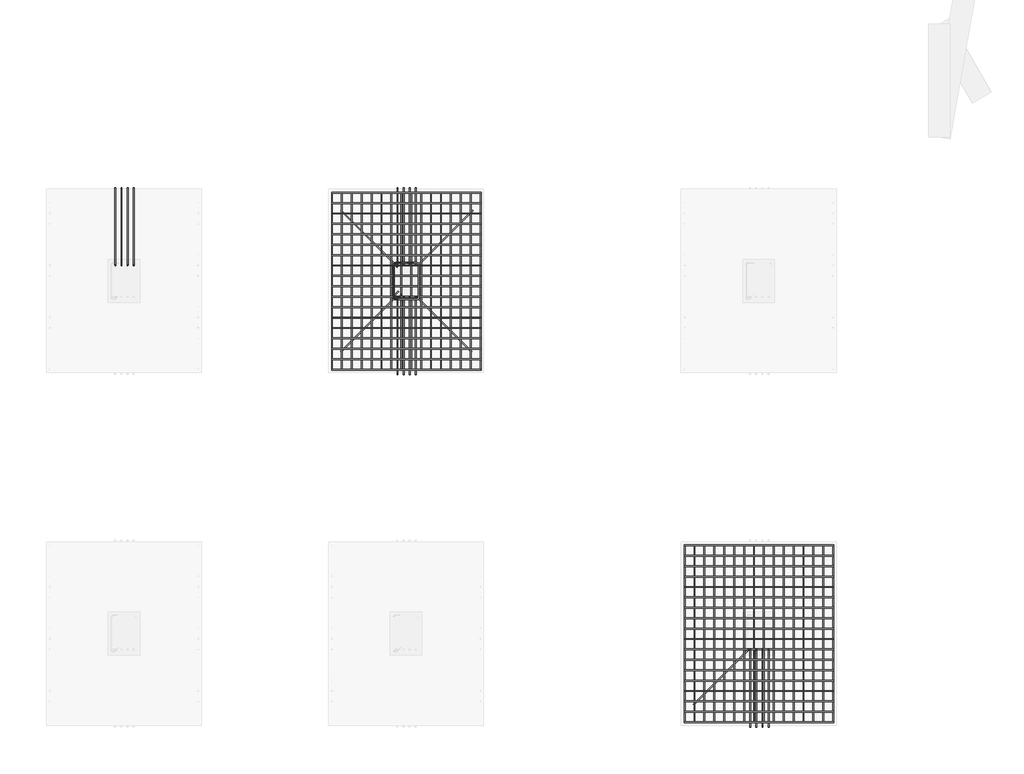
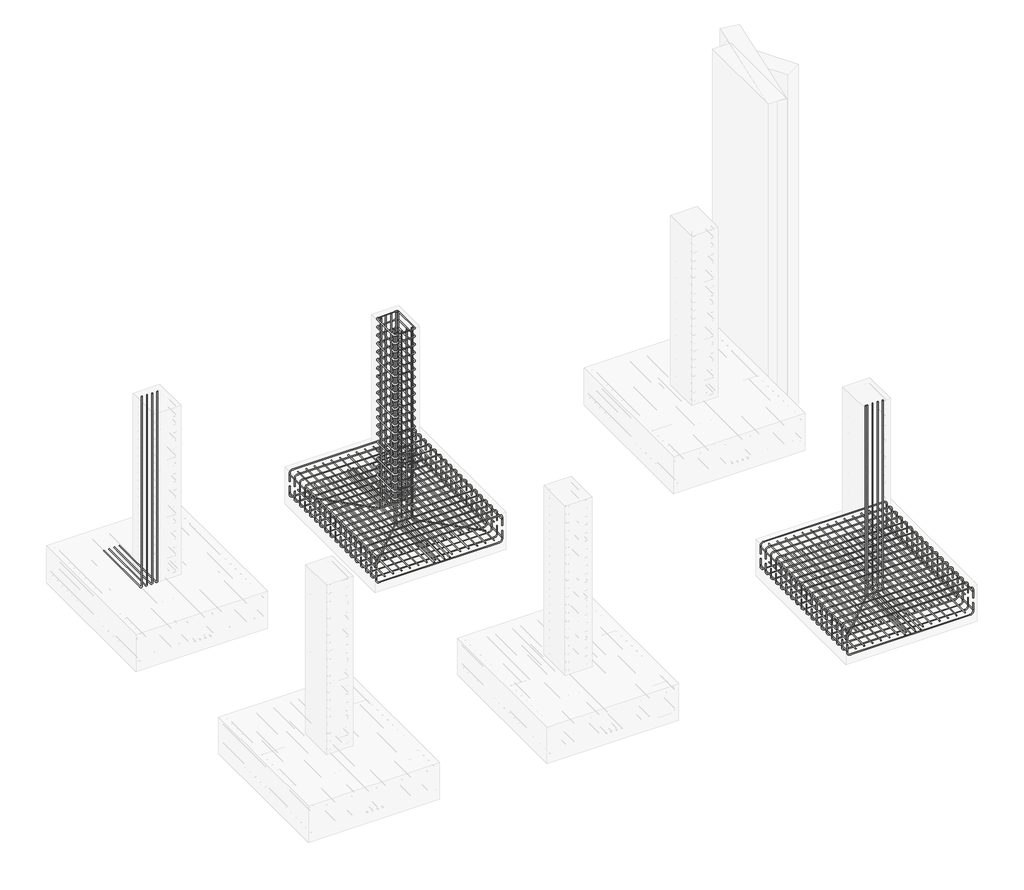
# One storey, part 15 of 33: 18 reinforcing bars.
"""IFC4 building model written with IfcOpenShell, lengths in millimetres."""

from ifc_helpers import new_model, si_unit, point, frame, origin, place, context, project, spatial, polyline, circle_curve, trimmed, segment, composite_curve, source, transform, mapped, element, save
from ifc_brep_helpers import swept_disk

model = new_model("IFC4")

# Units and contexts
model_context = context("Model", 3, world=origin())
ifc_project = project(units=[si_unit("LENGTHUNIT", "METRE", prefix="MILLI")], contexts=[model_context])

# Site, building, storey
site = spatial("IfcSite", under=ifc_project)
building = spatial("IfcBuilding", under=site)
storey = spatial("IfcBuildingStorey", under=building, Elevation=-3000.0)

# Reinforcing bars
placement = place(None, origin())
reinforcing_bar_shape = source(origin(), model_context, "Body", "SolidModel", [
    swept_disk(composite_curve([segment(polyline([(-5693.4642742, 2955.9391866, -3240.0), (-5693.4642742, 2955.9391866, -3092.7)]), True, "CONTINUOUS"), segment(trimmed(circle_curve(frame((-5647.1142742, 2955.9391866, -3092.7), z_axis=(0.0, 1.0, 0.0), x_axis=(-46.349999999999454, 0.0, 0.0)), 46.35), [point((-5693.4642742, 2955.9391866, -3092.7))], [point((-5647.1142742, 2955.9391866, -3046.35))], True, "CARTESIAN"), True, "CONTINUOUS"), segment(polyline([(-5647.1142742, 2955.9391866, -3046.35), (-3632.5142742, 2955.9391866, -3046.35)]), True, "CONTINUOUS"), segment(trimmed(circle_curve(frame((-3632.5142742, 2955.9391866, -3092.7), z_axis=(0.0, 1.0, 0.0), x_axis=(0.0, 0.0, 46.34999999999991)), 46.35), [point((-3632.5142742, 2955.9391866, -3046.35))], [point((-3586.1642742, 2955.9391866, -3092.7))], True, "CARTESIAN"), True, "CONTINUOUS"), segment(polyline([(-3586.1642742, 2955.9391866, -3092.7), (-3586.1642742, 2955.9391866, -3240.0)]), True, "CONTINUOUS")], self_intersect=False), 6.35),
])
element("IfcReinforcingBar", 1, at=placement, inside=storey, context=model_context, shape_type="MappedRepresentation", body=[
    mapped(reinforcing_bar_shape, transform((0.0, 0.0, 0.0), x_axis=(1.0, 0.0, 0.0), y_axis=(0.0, 1.0, 0.0), z_axis=(0.0, 0.0, 1.0))),
    mapped(reinforcing_bar_shape, transform((0.0, -147.4882353, 0.0), x_axis=(1.0, 0.0, 0.0), y_axis=(0.0, 1.0, 0.0), z_axis=(0.0, 0.0, 1.0))),
    mapped(reinforcing_bar_shape, transform((0.0, -294.9764706, 0.0), x_axis=(1.0, 0.0, 0.0), y_axis=(0.0, 1.0, 0.0), z_axis=(0.0, 0.0, 1.0))),
    mapped(reinforcing_bar_shape, transform((0.0, -442.4647059, 0.0), x_axis=(1.0, 0.0, 0.0), y_axis=(0.0, 1.0, 0.0), z_axis=(0.0, 0.0, 1.0))),
    mapped(reinforcing_bar_shape, transform((0.0, -589.9529412, 0.0), x_axis=(1.0, 0.0, 0.0), y_axis=(0.0, 1.0, 0.0), z_axis=(0.0, 0.0, 1.0))),
    mapped(reinforcing_bar_shape, transform((0.0, -737.4411765, 0.0), x_axis=(1.0, 0.0, 0.0), y_axis=(0.0, 1.0, 0.0), z_axis=(0.0, 0.0, 1.0))),
    mapped(reinforcing_bar_shape, transform((0.0, -884.9294118, 0.0), x_axis=(1.0, 0.0, 0.0), y_axis=(0.0, 1.0, 0.0), z_axis=(0.0, 0.0, 1.0))),
    mapped(reinforcing_bar_shape, transform((0.0, -1032.4176471, 0.0), x_axis=(1.0, 0.0, 0.0), y_axis=(0.0, 1.0, 0.0), z_axis=(0.0, 0.0, 1.0))),
    mapped(reinforcing_bar_shape, transform((0.0, -1179.9058824, 0.0), x_axis=(1.0, 0.0, 0.0), y_axis=(0.0, 1.0, 0.0), z_axis=(0.0, 0.0, 1.0))),
    mapped(reinforcing_bar_shape, transform((0.0, -1327.3941176, 0.0), x_axis=(1.0, 0.0, 0.0), y_axis=(0.0, 1.0, 0.0), z_axis=(0.0, 0.0, 1.0))),
    mapped(reinforcing_bar_shape, transform((0.0, -1474.8823529, 0.0), x_axis=(1.0, 0.0, 0.0), y_axis=(0.0, 1.0, 0.0), z_axis=(0.0, 0.0, 1.0))),
    mapped(reinforcing_bar_shape, transform((0.0, -1622.3705882, 0.0), x_axis=(1.0, 0.0, 0.0), y_axis=(0.0, 1.0, 0.0), z_axis=(0.0, 0.0, 1.0))),
    mapped(reinforcing_bar_shape, transform((0.0, -1769.8588235, 0.0), x_axis=(1.0, 0.0, 0.0), y_axis=(0.0, 1.0, 0.0), z_axis=(0.0, 0.0, 1.0))),
    mapped(reinforcing_bar_shape, transform((0.0, -1917.3470588, 0.0), x_axis=(1.0, 0.0, 0.0), y_axis=(0.0, 1.0, 0.0), z_axis=(0.0, 0.0, 1.0))),
    mapped(reinforcing_bar_shape, transform((0.0, -2064.8352941, 0.0), x_axis=(1.0, 0.0, 0.0), y_axis=(0.0, 1.0, 0.0), z_axis=(0.0, 0.0, 1.0))),
    mapped(reinforcing_bar_shape, transform((0.0, -2212.3235294, 0.0), x_axis=(1.0, 0.0, 0.0), y_axis=(0.0, 1.0, 0.0), z_axis=(0.0, 0.0, 1.0))),
    mapped(reinforcing_bar_shape, transform((0.0, -2359.8117647, 0.0), x_axis=(1.0, 0.0, 0.0), y_axis=(0.0, 1.0, 0.0), z_axis=(0.0, 0.0, 1.0))),
    mapped(reinforcing_bar_shape, transform((0.0, -2507.3, 0.0), x_axis=(1.0, 0.0, 0.0), y_axis=(0.0, 1.0, 0.0), z_axis=(0.0, 0.0, 1.0))),
])
reinforcing_bar_2_shape = source(origin(), model_context, "Body", "SolidModel", [
    swept_disk(composite_curve([segment(polyline([(-3586.1642742, 2955.9391866, -3330.080452), (-3586.1642742, 2955.9391866, -3477.380452)]), True, "CONTINUOUS"), segment(trimmed(circle_curve(frame((-3632.5142742, 2955.9391866, -3477.380452), z_axis=(0.0, 1.0, 0.0), x_axis=(46.34999999999991, 0.0, 0.0)), 46.35), [point((-3586.1642742, 2955.9391866, -3477.380452))], [point((-3632.5142742, 2955.9391866, -3523.730452))], True, "CARTESIAN"), True, "CONTINUOUS"), segment(polyline([(-3632.5142742, 2955.9391866, -3523.730452), (-5647.1142742, 2955.9391866, -3523.730452)]), True, "CONTINUOUS"), segment(trimmed(circle_curve(frame((-5647.1142742, 2955.9391866, -3477.380452), z_axis=(0.0, 1.0, 0.0), x_axis=(0.0, 0.0, -46.34999999999991)), 46.35), [point((-5647.1142742, 2955.9391866, -3523.730452))], [point((-5693.4642742, 2955.9391866, -3477.380452))], True, "CARTESIAN"), True, "CONTINUOUS"), segment(polyline([(-5693.4642742, 2955.9391866, -3477.380452), (-5693.4642742, 2955.9391866, -3330.080452)]), True, "CONTINUOUS")], self_intersect=False), 6.35),
])
element("IfcReinforcingBar", 2, at=placement, inside=storey, context=model_context, shape_type="MappedRepresentation", body=[
    mapped(reinforcing_bar_2_shape, transform((0.0, 0.0, 0.0), x_axis=(1.0, 0.0, 0.0), y_axis=(0.0, 1.0, 0.0), z_axis=(0.0, 0.0, 1.0))),
    mapped(reinforcing_bar_2_shape, transform((0.0, -147.4882353, 0.0), x_axis=(1.0, 0.0, 0.0), y_axis=(0.0, 1.0, 0.0), z_axis=(0.0, 0.0, 1.0))),
    mapped(reinforcing_bar_2_shape, transform((0.0, -294.9764706, 0.0), x_axis=(1.0, 0.0, 0.0), y_axis=(0.0, 1.0, 0.0), z_axis=(0.0, 0.0, 1.0))),
    mapped(reinforcing_bar_2_shape, transform((0.0, -442.4647059, 0.0), x_axis=(1.0, 0.0, 0.0), y_axis=(0.0, 1.0, 0.0), z_axis=(0.0, 0.0, 1.0))),
    mapped(reinforcing_bar_2_shape, transform((0.0, -589.9529412, 0.0), x_axis=(1.0, 0.0, 0.0), y_axis=(0.0, 1.0, 0.0), z_axis=(0.0, 0.0, 1.0))),
    mapped(reinforcing_bar_2_shape, transform((0.0, -737.4411765, 0.0), x_axis=(1.0, 0.0, 0.0), y_axis=(0.0, 1.0, 0.0), z_axis=(0.0, 0.0, 1.0))),
    mapped(reinforcing_bar_2_shape, transform((0.0, -884.9294118, 0.0), x_axis=(1.0, 0.0, 0.0), y_axis=(0.0, 1.0, 0.0), z_axis=(0.0, 0.0, 1.0))),
    mapped(reinforcing_bar_2_shape, transform((0.0, -1032.4176471, 0.0), x_axis=(1.0, 0.0, 0.0), y_axis=(0.0, 1.0, 0.0), z_axis=(0.0, 0.0, 1.0))),
    mapped(reinforcing_bar_2_shape, transform((0.0, -1179.9058824, 0.0), x_axis=(1.0, 0.0, 0.0), y_axis=(0.0, 1.0, 0.0), z_axis=(0.0, 0.0, 1.0))),
    mapped(reinforcing_bar_2_shape, transform((0.0, -1327.3941176, 0.0), x_axis=(1.0, 0.0, 0.0), y_axis=(0.0, 1.0, 0.0), z_axis=(0.0, 0.0, 1.0))),
    mapped(reinforcing_bar_2_shape, transform((0.0, -1474.8823529, 0.0), x_axis=(1.0, 0.0, 0.0), y_axis=(0.0, 1.0, 0.0), z_axis=(0.0, 0.0, 1.0))),
    mapped(reinforcing_bar_2_shape, transform((0.0, -1622.3705882, 0.0), x_axis=(1.0, 0.0, 0.0), y_axis=(0.0, 1.0, 0.0), z_axis=(0.0, 0.0, 1.0))),
    mapped(reinforcing_bar_2_shape, transform((0.0, -1769.8588235, 0.0), x_axis=(1.0, 0.0, 0.0), y_axis=(0.0, 1.0, 0.0), z_axis=(0.0, 0.0, 1.0))),
    mapped(reinforcing_bar_2_shape, transform((0.0, -1917.3470588, 0.0), x_axis=(1.0, 0.0, 0.0), y_axis=(0.0, 1.0, 0.0), z_axis=(0.0, 0.0, 1.0))),
    mapped(reinforcing_bar_2_shape, transform((0.0, -2064.8352941, 0.0), x_axis=(1.0, 0.0, 0.0), y_axis=(0.0, 1.0, 0.0), z_axis=(0.0, 0.0, 1.0))),
    mapped(reinforcing_bar_2_shape, transform((0.0, -2212.3235294, 0.0), x_axis=(1.0, 0.0, 0.0), y_axis=(0.0, 1.0, 0.0), z_axis=(0.0, 0.0, 1.0))),
    mapped(reinforcing_bar_2_shape, transform((0.0, -2359.8117647, 0.0), x_axis=(1.0, 0.0, 0.0), y_axis=(0.0, 1.0, 0.0), z_axis=(0.0, 0.0, 1.0))),
    mapped(reinforcing_bar_2_shape, transform((0.0, -2507.3, 0.0), x_axis=(1.0, 0.0, 0.0), y_axis=(0.0, 1.0, 0.0), z_axis=(0.0, 0.0, 1.0))),
])
reinforcing_bar_3_shape = source(origin(), model_context, "Body", "SolidModel", [
    swept_disk(composite_curve([segment(polyline([(-3586.1642742, 442.2891866, -3447.8614173), (-3586.1642742, 2962.2891866, -3447.8614173)]), True, "CONTINUOUS")], self_intersect=False), 6.35),
])
element("IfcReinforcingBar", 3, at=placement, inside=storey, context=model_context, shape_type="MappedRepresentation", body=[
    mapped(reinforcing_bar_3_shape, transform((0.0, 0.0, 0.0), x_axis=(1.0, 0.0, 0.0), y_axis=(0.0, 1.0, 0.0), z_axis=(0.0, 0.0, 1.0))),
    mapped(reinforcing_bar_3_shape, transform((-140.4866667, 0.0, 0.0), x_axis=(1.0, 0.0, 0.0), y_axis=(0.0, 1.0, 0.0), z_axis=(0.0, 0.0, 1.0))),
    mapped(reinforcing_bar_3_shape, transform((-280.9733333, 0.0, 0.0), x_axis=(1.0, 0.0, 0.0), y_axis=(0.0, 1.0, 0.0), z_axis=(0.0, 0.0, 1.0))),
    mapped(reinforcing_bar_3_shape, transform((-421.46, 0.0, 0.0), x_axis=(1.0, 0.0, 0.0), y_axis=(0.0, 1.0, 0.0), z_axis=(0.0, 0.0, 1.0))),
    mapped(reinforcing_bar_3_shape, transform((-561.9466667, 0.0, 0.0), x_axis=(1.0, 0.0, 0.0), y_axis=(0.0, 1.0, 0.0), z_axis=(0.0, 0.0, 1.0))),
    mapped(reinforcing_bar_3_shape, transform((-702.4333333, 0.0, 0.0), x_axis=(1.0, 0.0, 0.0), y_axis=(0.0, 1.0, 0.0), z_axis=(0.0, 0.0, 1.0))),
    mapped(reinforcing_bar_3_shape, transform((-842.92, 0.0, 0.0), x_axis=(1.0, 0.0, 0.0), y_axis=(0.0, 1.0, 0.0), z_axis=(0.0, 0.0, 1.0))),
    mapped(reinforcing_bar_3_shape, transform((-983.4066667, 0.0, 0.0), x_axis=(1.0, 0.0, 0.0), y_axis=(0.0, 1.0, 0.0), z_axis=(0.0, 0.0, 1.0))),
    mapped(reinforcing_bar_3_shape, transform((-1123.8933333, 0.0, 0.0), x_axis=(1.0, 0.0, 0.0), y_axis=(0.0, 1.0, 0.0), z_axis=(0.0, 0.0, 1.0))),
    mapped(reinforcing_bar_3_shape, transform((-1264.38, 0.0, 0.0), x_axis=(1.0, 0.0, 0.0), y_axis=(0.0, 1.0, 0.0), z_axis=(0.0, 0.0, 1.0))),
    mapped(reinforcing_bar_3_shape, transform((-1404.8666667, 0.0, 0.0), x_axis=(1.0, 0.0, 0.0), y_axis=(0.0, 1.0, 0.0), z_axis=(0.0, 0.0, 1.0))),
    mapped(reinforcing_bar_3_shape, transform((-1545.3533333, 0.0, 0.0), x_axis=(1.0, 0.0, 0.0), y_axis=(0.0, 1.0, 0.0), z_axis=(0.0, 0.0, 1.0))),
    mapped(reinforcing_bar_3_shape, transform((-1685.84, 0.0, 0.0), x_axis=(1.0, 0.0, 0.0), y_axis=(0.0, 1.0, 0.0), z_axis=(0.0, 0.0, 1.0))),
    mapped(reinforcing_bar_3_shape, transform((-1826.3266667, 0.0, 0.0), x_axis=(1.0, 0.0, 0.0), y_axis=(0.0, 1.0, 0.0), z_axis=(0.0, 0.0, 1.0))),
    mapped(reinforcing_bar_3_shape, transform((-1966.8133333, 0.0, 0.0), x_axis=(1.0, 0.0, 0.0), y_axis=(0.0, 1.0, 0.0), z_axis=(0.0, 0.0, 1.0))),
    mapped(reinforcing_bar_3_shape, transform((-2107.3, 0.0, 0.0), x_axis=(1.0, 0.0, 0.0), y_axis=(0.0, 1.0, 0.0), z_axis=(0.0, 0.0, 1.0))),
])
reinforcing_bar_4_shape = source(origin(), model_context, "Body", "SolidModel", [
    swept_disk(composite_curve([segment(polyline([(-5693.4642742, 442.2891866, -3122.7084113), (-5693.4642742, 2962.2891866, -3122.7084113)]), True, "CONTINUOUS")], self_intersect=False), 6.35),
])
element("IfcReinforcingBar", 4, at=placement, inside=storey, context=model_context, shape_type="MappedRepresentation", body=[
    mapped(reinforcing_bar_4_shape, transform((0.0, 0.0, 0.0), x_axis=(1.0, 0.0, 0.0), y_axis=(0.0, 1.0, 0.0), z_axis=(0.0, 0.0, 1.0))),
    mapped(reinforcing_bar_4_shape, transform((140.4866667, 0.0, 0.0), x_axis=(1.0, 0.0, 0.0), y_axis=(0.0, 1.0, 0.0), z_axis=(0.0, 0.0, 1.0))),
    mapped(reinforcing_bar_4_shape, transform((280.9733333, 0.0, 0.0), x_axis=(1.0, 0.0, 0.0), y_axis=(0.0, 1.0, 0.0), z_axis=(0.0, 0.0, 1.0))),
    mapped(reinforcing_bar_4_shape, transform((421.46, 0.0, 0.0), x_axis=(1.0, 0.0, 0.0), y_axis=(0.0, 1.0, 0.0), z_axis=(0.0, 0.0, 1.0))),
    mapped(reinforcing_bar_4_shape, transform((561.9466667, 0.0, 0.0), x_axis=(1.0, 0.0, 0.0), y_axis=(0.0, 1.0, 0.0), z_axis=(0.0, 0.0, 1.0))),
    mapped(reinforcing_bar_4_shape, transform((702.4333333, 0.0, 0.0), x_axis=(1.0, 0.0, 0.0), y_axis=(0.0, 1.0, 0.0), z_axis=(0.0, 0.0, 1.0))),
    mapped(reinforcing_bar_4_shape, transform((842.92, 0.0, 0.0), x_axis=(1.0, 0.0, 0.0), y_axis=(0.0, 1.0, 0.0), z_axis=(0.0, 0.0, 1.0))),
    mapped(reinforcing_bar_4_shape, transform((983.4066667, 0.0, 0.0), x_axis=(1.0, 0.0, 0.0), y_axis=(0.0, 1.0, 0.0), z_axis=(0.0, 0.0, 1.0))),
    mapped(reinforcing_bar_4_shape, transform((1123.8933333, 0.0, 0.0), x_axis=(1.0, 0.0, 0.0), y_axis=(0.0, 1.0, 0.0), z_axis=(0.0, 0.0, 1.0))),
    mapped(reinforcing_bar_4_shape, transform((1264.38, 0.0, 0.0), x_axis=(1.0, 0.0, 0.0), y_axis=(0.0, 1.0, 0.0), z_axis=(0.0, 0.0, 1.0))),
    mapped(reinforcing_bar_4_shape, transform((1404.8666667, 0.0, 0.0), x_axis=(1.0, 0.0, 0.0), y_axis=(0.0, 1.0, 0.0), z_axis=(0.0, 0.0, 1.0))),
    mapped(reinforcing_bar_4_shape, transform((1545.3533333, 0.0, 0.0), x_axis=(1.0, 0.0, 0.0), y_axis=(0.0, 1.0, 0.0), z_axis=(0.0, 0.0, 1.0))),
    mapped(reinforcing_bar_4_shape, transform((1685.84, 0.0, 0.0), x_axis=(1.0, 0.0, 0.0), y_axis=(0.0, 1.0, 0.0), z_axis=(0.0, 0.0, 1.0))),
    mapped(reinforcing_bar_4_shape, transform((1826.3266667, 0.0, 0.0), x_axis=(1.0, 0.0, 0.0), y_axis=(0.0, 1.0, 0.0), z_axis=(0.0, 0.0, 1.0))),
    mapped(reinforcing_bar_4_shape, transform((1966.8133333, 0.0, 0.0), x_axis=(1.0, 0.0, 0.0), y_axis=(0.0, 1.0, 0.0), z_axis=(0.0, 0.0, 1.0))),
    mapped(reinforcing_bar_4_shape, transform((2107.3, 0.0, 0.0), x_axis=(1.0, 0.0, 0.0), y_axis=(0.0, 1.0, 0.0), z_axis=(0.0, 0.0, 1.0))),
])
reinforcing_bar_5_shape = source(origin(), model_context, "Body", "SolidModel", [
    swept_disk(composite_curve([segment(polyline([(-10693.4642742, 7955.9391866, -3240.0), (-10693.4642742, 7955.9391866, -3092.7)]), True, "CONTINUOUS"), segment(trimmed(circle_curve(frame((-10647.1142742, 7955.9391866, -3092.7), z_axis=(0.0, 1.0, 0.0), x_axis=(-46.350000000000364, 0.0, 0.0)), 46.35), [point((-10693.4642742, 7955.9391866, -3092.7))], [point((-10647.1142742, 7955.9391866, -3046.35))], True, "CARTESIAN"), True, "CONTINUOUS"), segment(polyline([(-10647.1142742, 7955.9391866, -3046.35), (-8632.5142742, 7955.9391866, -3046.35)]), True, "CONTINUOUS"), segment(trimmed(circle_curve(frame((-8632.5142742, 7955.9391866, -3092.7), z_axis=(0.0, 1.0, 0.0), x_axis=(0.0, 0.0, 46.34999999999991)), 46.35), [point((-8632.5142742, 7955.9391866, -3046.35))], [point((-8586.1642742, 7955.9391866, -3092.7))], True, "CARTESIAN"), True, "CONTINUOUS"), segment(polyline([(-8586.1642742, 7955.9391866, -3092.7), (-8586.1642742, 7955.9391866, -3240.0)]), True, "CONTINUOUS")], self_intersect=False), 6.35),
])
element("IfcReinforcingBar", 5, at=placement, inside=storey, context=model_context, shape_type="MappedRepresentation", body=[
    mapped(reinforcing_bar_5_shape, transform((0.0, 0.0, 0.0), x_axis=(1.0, 0.0, 0.0), y_axis=(0.0, 1.0, 0.0), z_axis=(0.0, 0.0, 1.0))),
    mapped(reinforcing_bar_5_shape, transform((0.0, -147.4882353, 0.0), x_axis=(1.0, 0.0, 0.0), y_axis=(0.0, 1.0, 0.0), z_axis=(0.0, 0.0, 1.0))),
    mapped(reinforcing_bar_5_shape, transform((0.0, -294.9764706, 0.0), x_axis=(1.0, 0.0, 0.0), y_axis=(0.0, 1.0, 0.0), z_axis=(0.0, 0.0, 1.0))),
    mapped(reinforcing_bar_5_shape, transform((0.0, -442.4647059, 0.0), x_axis=(1.0, 0.0, 0.0), y_axis=(0.0, 1.0, 0.0), z_axis=(0.0, 0.0, 1.0))),
    mapped(reinforcing_bar_5_shape, transform((0.0, -589.9529412, 0.0), x_axis=(1.0, 0.0, 0.0), y_axis=(0.0, 1.0, 0.0), z_axis=(0.0, 0.0, 1.0))),
    mapped(reinforcing_bar_5_shape, transform((0.0, -737.4411765, 0.0), x_axis=(1.0, 0.0, 0.0), y_axis=(0.0, 1.0, 0.0), z_axis=(0.0, 0.0, 1.0))),
    mapped(reinforcing_bar_5_shape, transform((0.0, -884.9294118, 0.0), x_axis=(1.0, 0.0, 0.0), y_axis=(0.0, 1.0, 0.0), z_axis=(0.0, 0.0, 1.0))),
    mapped(reinforcing_bar_5_shape, transform((0.0, -1032.4176471, 0.0), x_axis=(1.0, 0.0, 0.0), y_axis=(0.0, 1.0, 0.0), z_axis=(0.0, 0.0, 1.0))),
    mapped(reinforcing_bar_5_shape, transform((0.0, -1179.9058824, 0.0), x_axis=(1.0, 0.0, 0.0), y_axis=(0.0, 1.0, 0.0), z_axis=(0.0, 0.0, 1.0))),
    mapped(reinforcing_bar_5_shape, transform((0.0, -1327.3941176, 0.0), x_axis=(1.0, 0.0, 0.0), y_axis=(0.0, 1.0, 0.0), z_axis=(0.0, 0.0, 1.0))),
    mapped(reinforcing_bar_5_shape, transform((0.0, -1474.8823529, 0.0), x_axis=(1.0, 0.0, 0.0), y_axis=(0.0, 1.0, 0.0), z_axis=(0.0, 0.0, 1.0))),
    mapped(reinforcing_bar_5_shape, transform((0.0, -1622.3705882, 0.0), x_axis=(1.0, 0.0, 0.0), y_axis=(0.0, 1.0, 0.0), z_axis=(0.0, 0.0, 1.0))),
    mapped(reinforcing_bar_5_shape, transform((0.0, -1769.8588235, 0.0), x_axis=(1.0, 0.0, 0.0), y_axis=(0.0, 1.0, 0.0), z_axis=(0.0, 0.0, 1.0))),
    mapped(reinforcing_bar_5_shape, transform((0.0, -1917.3470588, 0.0), x_axis=(1.0, 0.0, 0.0), y_axis=(0.0, 1.0, 0.0), z_axis=(0.0, 0.0, 1.0))),
    mapped(reinforcing_bar_5_shape, transform((0.0, -2064.8352941, 0.0), x_axis=(1.0, 0.0, 0.0), y_axis=(0.0, 1.0, 0.0), z_axis=(0.0, 0.0, 1.0))),
    mapped(reinforcing_bar_5_shape, transform((0.0, -2212.3235294, 0.0), x_axis=(1.0, 0.0, 0.0), y_axis=(0.0, 1.0, 0.0), z_axis=(0.0, 0.0, 1.0))),
    mapped(reinforcing_bar_5_shape, transform((0.0, -2359.8117647, 0.0), x_axis=(1.0, 0.0, 0.0), y_axis=(0.0, 1.0, 0.0), z_axis=(0.0, 0.0, 1.0))),
    mapped(reinforcing_bar_5_shape, transform((0.0, -2507.3, 0.0), x_axis=(1.0, 0.0, 0.0), y_axis=(0.0, 1.0, 0.0), z_axis=(0.0, 0.0, 1.0))),
])
reinforcing_bar_6_shape = source(origin(), model_context, "Body", "SolidModel", [
    swept_disk(composite_curve([segment(polyline([(-8586.1642742, 7955.9391866, -3330.080452), (-8586.1642742, 7955.9391866, -3477.380452)]), True, "CONTINUOUS"), segment(trimmed(circle_curve(frame((-8632.5142742, 7955.9391866, -3477.380452), z_axis=(0.0, 1.0, 0.0), x_axis=(46.350000000000364, 0.0, 0.0)), 46.35), [point((-8586.1642742, 7955.9391866, -3477.380452))], [point((-8632.5142742, 7955.9391866, -3523.730452))], True, "CARTESIAN"), True, "CONTINUOUS"), segment(polyline([(-8632.5142742, 7955.9391866, -3523.730452), (-10647.1142742, 7955.9391866, -3523.730452)]), True, "CONTINUOUS"), segment(trimmed(circle_curve(frame((-10647.1142742, 7955.9391866, -3477.380452), z_axis=(0.0, 1.0, 0.0), x_axis=(0.0, 0.0, -46.34999999999991)), 46.35), [point((-10647.1142742, 7955.9391866, -3523.730452))], [point((-10693.4642742, 7955.9391866, -3477.380452))], True, "CARTESIAN"), True, "CONTINUOUS"), segment(polyline([(-10693.4642742, 7955.9391866, -3477.380452), (-10693.4642742, 7955.9391866, -3330.080452)]), True, "CONTINUOUS")], self_intersect=False), 6.35),
])
element("IfcReinforcingBar", 6, at=placement, inside=storey, context=model_context, shape_type="MappedRepresentation", body=[
    mapped(reinforcing_bar_6_shape, transform((0.0, 0.0, 0.0), x_axis=(1.0, 0.0, 0.0), y_axis=(0.0, 1.0, 0.0), z_axis=(0.0, 0.0, 1.0))),
    mapped(reinforcing_bar_6_shape, transform((0.0, -147.4882353, 0.0), x_axis=(1.0, 0.0, 0.0), y_axis=(0.0, 1.0, 0.0), z_axis=(0.0, 0.0, 1.0))),
    mapped(reinforcing_bar_6_shape, transform((0.0, -294.9764706, 0.0), x_axis=(1.0, 0.0, 0.0), y_axis=(0.0, 1.0, 0.0), z_axis=(0.0, 0.0, 1.0))),
    mapped(reinforcing_bar_6_shape, transform((0.0, -442.4647059, 0.0), x_axis=(1.0, 0.0, 0.0), y_axis=(0.0, 1.0, 0.0), z_axis=(0.0, 0.0, 1.0))),
    mapped(reinforcing_bar_6_shape, transform((0.0, -589.9529412, 0.0), x_axis=(1.0, 0.0, 0.0), y_axis=(0.0, 1.0, 0.0), z_axis=(0.0, 0.0, 1.0))),
    mapped(reinforcing_bar_6_shape, transform((0.0, -737.4411765, 0.0), x_axis=(1.0, 0.0, 0.0), y_axis=(0.0, 1.0, 0.0), z_axis=(0.0, 0.0, 1.0))),
    mapped(reinforcing_bar_6_shape, transform((0.0, -884.9294118, 0.0), x_axis=(1.0, 0.0, 0.0), y_axis=(0.0, 1.0, 0.0), z_axis=(0.0, 0.0, 1.0))),
    mapped(reinforcing_bar_6_shape, transform((0.0, -1032.4176471, 0.0), x_axis=(1.0, 0.0, 0.0), y_axis=(0.0, 1.0, 0.0), z_axis=(0.0, 0.0, 1.0))),
    mapped(reinforcing_bar_6_shape, transform((0.0, -1179.9058824, 0.0), x_axis=(1.0, 0.0, 0.0), y_axis=(0.0, 1.0, 0.0), z_axis=(0.0, 0.0, 1.0))),
    mapped(reinforcing_bar_6_shape, transform((0.0, -1327.3941176, 0.0), x_axis=(1.0, 0.0, 0.0), y_axis=(0.0, 1.0, 0.0), z_axis=(0.0, 0.0, 1.0))),
    mapped(reinforcing_bar_6_shape, transform((0.0, -1474.8823529, 0.0), x_axis=(1.0, 0.0, 0.0), y_axis=(0.0, 1.0, 0.0), z_axis=(0.0, 0.0, 1.0))),
    mapped(reinforcing_bar_6_shape, transform((0.0, -1622.3705882, 0.0), x_axis=(1.0, 0.0, 0.0), y_axis=(0.0, 1.0, 0.0), z_axis=(0.0, 0.0, 1.0))),
    mapped(reinforcing_bar_6_shape, transform((0.0, -1769.8588235, 0.0), x_axis=(1.0, 0.0, 0.0), y_axis=(0.0, 1.0, 0.0), z_axis=(0.0, 0.0, 1.0))),
    mapped(reinforcing_bar_6_shape, transform((0.0, -1917.3470588, 0.0), x_axis=(1.0, 0.0, 0.0), y_axis=(0.0, 1.0, 0.0), z_axis=(0.0, 0.0, 1.0))),
    mapped(reinforcing_bar_6_shape, transform((0.0, -2064.8352941, 0.0), x_axis=(1.0, 0.0, 0.0), y_axis=(0.0, 1.0, 0.0), z_axis=(0.0, 0.0, 1.0))),
    mapped(reinforcing_bar_6_shape, transform((0.0, -2212.3235294, 0.0), x_axis=(1.0, 0.0, 0.0), y_axis=(0.0, 1.0, 0.0), z_axis=(0.0, 0.0, 1.0))),
    mapped(reinforcing_bar_6_shape, transform((0.0, -2359.8117647, 0.0), x_axis=(1.0, 0.0, 0.0), y_axis=(0.0, 1.0, 0.0), z_axis=(0.0, 0.0, 1.0))),
    mapped(reinforcing_bar_6_shape, transform((0.0, -2507.3, 0.0), x_axis=(1.0, 0.0, 0.0), y_axis=(0.0, 1.0, 0.0), z_axis=(0.0, 0.0, 1.0))),
])
reinforcing_bar_7_shape = source(origin(), model_context, "Body", "SolidModel", [
    swept_disk(composite_curve([segment(polyline([(-8586.1642742, 5442.2891866, -3447.8614173), (-8586.1642742, 7962.2891866, -3447.8614173)]), True, "CONTINUOUS")], self_intersect=False), 6.35),
])
element("IfcReinforcingBar", 7, at=placement, inside=storey, context=model_context, shape_type="MappedRepresentation", body=[
    mapped(reinforcing_bar_7_shape, transform((0.0, 0.0, 0.0), x_axis=(1.0, 0.0, 0.0), y_axis=(0.0, 1.0, 0.0), z_axis=(0.0, 0.0, 1.0))),
    mapped(reinforcing_bar_7_shape, transform((-140.4866667, 0.0, 0.0), x_axis=(1.0, 0.0, 0.0), y_axis=(0.0, 1.0, 0.0), z_axis=(0.0, 0.0, 1.0))),
    mapped(reinforcing_bar_7_shape, transform((-280.9733333, 0.0, 0.0), x_axis=(1.0, 0.0, 0.0), y_axis=(0.0, 1.0, 0.0), z_axis=(0.0, 0.0, 1.0))),
    mapped(reinforcing_bar_7_shape, transform((-421.46, 0.0, 0.0), x_axis=(1.0, 0.0, 0.0), y_axis=(0.0, 1.0, 0.0), z_axis=(0.0, 0.0, 1.0))),
    mapped(reinforcing_bar_7_shape, transform((-561.9466667, 0.0, 0.0), x_axis=(1.0, 0.0, 0.0), y_axis=(0.0, 1.0, 0.0), z_axis=(0.0, 0.0, 1.0))),
    mapped(reinforcing_bar_7_shape, transform((-702.4333333, 0.0, 0.0), x_axis=(1.0, 0.0, 0.0), y_axis=(0.0, 1.0, 0.0), z_axis=(0.0, 0.0, 1.0))),
    mapped(reinforcing_bar_7_shape, transform((-842.92, 0.0, 0.0), x_axis=(1.0, 0.0, 0.0), y_axis=(0.0, 1.0, 0.0), z_axis=(0.0, 0.0, 1.0))),
    mapped(reinforcing_bar_7_shape, transform((-983.4066667, 0.0, 0.0), x_axis=(1.0, 0.0, 0.0), y_axis=(0.0, 1.0, 0.0), z_axis=(0.0, 0.0, 1.0))),
    mapped(reinforcing_bar_7_shape, transform((-1123.8933333, 0.0, 0.0), x_axis=(1.0, 0.0, 0.0), y_axis=(0.0, 1.0, 0.0), z_axis=(0.0, 0.0, 1.0))),
    mapped(reinforcing_bar_7_shape, transform((-1264.38, 0.0, 0.0), x_axis=(1.0, 0.0, 0.0), y_axis=(0.0, 1.0, 0.0), z_axis=(0.0, 0.0, 1.0))),
    mapped(reinforcing_bar_7_shape, transform((-1404.8666667, 0.0, 0.0), x_axis=(1.0, 0.0, 0.0), y_axis=(0.0, 1.0, 0.0), z_axis=(0.0, 0.0, 1.0))),
    mapped(reinforcing_bar_7_shape, transform((-1545.3533333, 0.0, 0.0), x_axis=(1.0, 0.0, 0.0), y_axis=(0.0, 1.0, 0.0), z_axis=(0.0, 0.0, 1.0))),
    mapped(reinforcing_bar_7_shape, transform((-1685.84, 0.0, 0.0), x_axis=(1.0, 0.0, 0.0), y_axis=(0.0, 1.0, 0.0), z_axis=(0.0, 0.0, 1.0))),
    mapped(reinforcing_bar_7_shape, transform((-1826.3266667, 0.0, 0.0), x_axis=(1.0, 0.0, 0.0), y_axis=(0.0, 1.0, 0.0), z_axis=(0.0, 0.0, 1.0))),
    mapped(reinforcing_bar_7_shape, transform((-1966.8133333, 0.0, 0.0), x_axis=(1.0, 0.0, 0.0), y_axis=(0.0, 1.0, 0.0), z_axis=(0.0, 0.0, 1.0))),
    mapped(reinforcing_bar_7_shape, transform((-2107.3, 0.0, 0.0), x_axis=(1.0, 0.0, 0.0), y_axis=(0.0, 1.0, 0.0), z_axis=(0.0, 0.0, 1.0))),
])
reinforcing_bar_8_shape = source(origin(), model_context, "Body", "SolidModel", [
    swept_disk(composite_curve([segment(polyline([(-10693.4642742, 5442.2891866, -3122.7084113), (-10693.4642742, 7962.2891866, -3122.7084113)]), True, "CONTINUOUS")], self_intersect=False), 6.35),
])
element("IfcReinforcingBar", 8, at=placement, inside=storey, context=model_context, shape_type="MappedRepresentation", body=[
    mapped(reinforcing_bar_8_shape, transform((0.0, 0.0, 0.0), x_axis=(1.0, 0.0, 0.0), y_axis=(0.0, 1.0, 0.0), z_axis=(0.0, 0.0, 1.0))),
    mapped(reinforcing_bar_8_shape, transform((140.4866667, 0.0, 0.0), x_axis=(1.0, 0.0, 0.0), y_axis=(0.0, 1.0, 0.0), z_axis=(0.0, 0.0, 1.0))),
    mapped(reinforcing_bar_8_shape, transform((280.9733333, 0.0, 0.0), x_axis=(1.0, 0.0, 0.0), y_axis=(0.0, 1.0, 0.0), z_axis=(0.0, 0.0, 1.0))),
    mapped(reinforcing_bar_8_shape, transform((421.46, 0.0, 0.0), x_axis=(1.0, 0.0, 0.0), y_axis=(0.0, 1.0, 0.0), z_axis=(0.0, 0.0, 1.0))),
    mapped(reinforcing_bar_8_shape, transform((561.9466667, 0.0, 0.0), x_axis=(1.0, 0.0, 0.0), y_axis=(0.0, 1.0, 0.0), z_axis=(0.0, 0.0, 1.0))),
    mapped(reinforcing_bar_8_shape, transform((702.4333333, 0.0, 0.0), x_axis=(1.0, 0.0, 0.0), y_axis=(0.0, 1.0, 0.0), z_axis=(0.0, 0.0, 1.0))),
    mapped(reinforcing_bar_8_shape, transform((842.92, 0.0, 0.0), x_axis=(1.0, 0.0, 0.0), y_axis=(0.0, 1.0, 0.0), z_axis=(0.0, 0.0, 1.0))),
    mapped(reinforcing_bar_8_shape, transform((983.4066667, 0.0, 0.0), x_axis=(1.0, 0.0, 0.0), y_axis=(0.0, 1.0, 0.0), z_axis=(0.0, 0.0, 1.0))),
    mapped(reinforcing_bar_8_shape, transform((1123.8933333, 0.0, 0.0), x_axis=(1.0, 0.0, 0.0), y_axis=(0.0, 1.0, 0.0), z_axis=(0.0, 0.0, 1.0))),
    mapped(reinforcing_bar_8_shape, transform((1264.38, 0.0, 0.0), x_axis=(1.0, 0.0, 0.0), y_axis=(0.0, 1.0, 0.0), z_axis=(0.0, 0.0, 1.0))),
    mapped(reinforcing_bar_8_shape, transform((1404.8666667, 0.0, 0.0), x_axis=(1.0, 0.0, 0.0), y_axis=(0.0, 1.0, 0.0), z_axis=(0.0, 0.0, 1.0))),
    mapped(reinforcing_bar_8_shape, transform((1545.3533333, 0.0, 0.0), x_axis=(1.0, 0.0, 0.0), y_axis=(0.0, 1.0, 0.0), z_axis=(0.0, 0.0, 1.0))),
    mapped(reinforcing_bar_8_shape, transform((1685.84, 0.0, 0.0), x_axis=(1.0, 0.0, 0.0), y_axis=(0.0, 1.0, 0.0), z_axis=(0.0, 0.0, 1.0))),
    mapped(reinforcing_bar_8_shape, transform((1826.3266667, 0.0, 0.0), x_axis=(1.0, 0.0, 0.0), y_axis=(0.0, 1.0, 0.0), z_axis=(0.0, 0.0, 1.0))),
    mapped(reinforcing_bar_8_shape, transform((1966.8133333, 0.0, 0.0), x_axis=(1.0, 0.0, 0.0), y_axis=(0.0, 1.0, 0.0), z_axis=(0.0, 0.0, 1.0))),
    mapped(reinforcing_bar_8_shape, transform((2107.3, 0.0, 0.0), x_axis=(1.0, 0.0, 0.0), y_axis=(0.0, 1.0, 0.0), z_axis=(0.0, 0.0, 1.0))),
])
reinforcing_bar_9_shape = source(origin(), model_context, "Body", "SolidModel", [
    swept_disk(composite_curve([segment(polyline([(-13763.8841678, 6928.0721866, -40.0), (-13763.8841678, 6928.0721866, -3393.65)]), True, "CONTINUOUS"), segment(trimmed(circle_curve(frame((-13763.8841678, 6974.4221866, -3393.65), z_axis=(1.0, 0.0, 0.0), x_axis=(0.0, -46.349999999999454, 0.0)), 46.35), [point((-13763.8841678, 6928.0721866, -3393.65))], [point((-13763.8841678, 6974.4221866, -3440.0))], True, "CARTESIAN"), True, "CONTINUOUS"), segment(polyline([(-13763.8841678, 6974.4221866, -3440.0), (-13763.8841678, 8028.0721866, -3440.0)]), True, "CONTINUOUS")], self_intersect=False), 6.35),
])
element("IfcReinforcingBar", 9, at=placement, inside=storey, context=model_context, shape_type="MappedRepresentation", body=[
    mapped(reinforcing_bar_9_shape, transform((0.0, 0.0, 0.0), x_axis=(1.0, 0.0, 0.0), y_axis=(0.0, 1.0, 0.0), z_axis=(0.0, 0.0, 1.0))),
    mapped(reinforcing_bar_9_shape, transform((86.8979716, 0.0, 0.0), x_axis=(1.0, 0.0, 0.0), y_axis=(0.0, 1.0, 0.0), z_axis=(0.0, 0.0, 1.0))),
    mapped(reinforcing_bar_9_shape, transform((173.7959432, 0.0, 0.0), x_axis=(1.0, 0.0, 0.0), y_axis=(0.0, 1.0, 0.0), z_axis=(0.0, 0.0, 1.0))),
    mapped(reinforcing_bar_9_shape, transform((260.6939148, 0.0, 0.0), x_axis=(1.0, 0.0, 0.0), y_axis=(0.0, 1.0, 0.0), z_axis=(0.0, 0.0, 1.0))),
])
reinforcing_bar_10_shape = source(origin(), model_context, "Body", "SolidModel", [
    swept_disk(composite_curve([segment(polyline([(-9753.5385089, 6553.1005472, -2953.65), (-9809.2820718, 6497.3569842, -2953.65)]), True, "CONTINUOUS"), segment(trimmed(circle_curve(frame((-9787.1142742, 6475.1891866, -2953.65), z_axis=(0.0, 0.0, 1.0), x_axis=(-22.167797600000995, 22.167797600000085, 0.0)), 31.35), [point((-9809.2820718, 6497.3569842, -2953.65))], [point((-9787.1142742, 6443.8391866, -2953.65))], True, "CARTESIAN"), True, "CONTINUOUS"), segment(polyline([(-9787.1142742, 6443.8391866, -2953.65), (-9492.5142742, 6443.8391866, -2953.65)]), True, "CONTINUOUS"), segment(trimmed(circle_curve(frame((-9492.5142742, 6475.1891866, -2953.65), z_axis=(0.0, 0.0, 1.0), x_axis=(0.0, -31.349999999999454, 0.0)), 31.35), [point((-9492.5142742, 6443.8391866, -2953.65))], [point((-9461.1642742, 6475.1891866, -2953.65))], True, "CARTESIAN"), True, "CONTINUOUS"), segment(polyline([(-9461.1642742, 6475.1891866, -2953.65), (-9461.1642742, 6929.3891866, -2953.65)]), True, "CONTINUOUS"), segment(trimmed(circle_curve(frame((-9492.4944891, 6929.3891866, -2954.7636125), z_axis=(-0.0355219283344822, 0.0, 0.9993688971583016), x_axis=(31.33021489999919, 0.0, 1.1136124999998174)), 31.35), [point((-9461.1642742, 6929.3891866, -2953.65))], [point((-9492.4944891, 6960.7391866, -2954.7636125))], True, "CARTESIAN"), True, "CONTINUOUS"), segment(polyline([(-9492.4944891, 6960.7391866, -2954.7636125), (-9787.1340593, 6960.7391866, -2965.2363875)]), True, "CONTINUOUS"), segment(trimmed(circle_curve(frame((-9787.1340593, 6929.3891866, -2965.2363875), z_axis=(-0.0355219283344822, 0.0, 0.9993688971583016), x_axis=(0.0, 31.349999999999454, 0.0)), 31.35), [point((-9787.1340593, 6960.7391866, -2965.2363875))], [point((-9818.4642742, 6929.3891866, -2966.35))], True, "CARTESIAN"), True, "CONTINUOUS"), segment(polyline([(-9818.4642742, 6929.3891866, -2966.35), (-9818.4642742, 6475.1891866, -2966.35)]), True, "CONTINUOUS"), segment(trimmed(circle_curve(frame((-9787.1142742, 6475.1891866, -2966.35), z_axis=(0.0, 0.0, 1.0), x_axis=(-31.350000000000364, 0.0, 0.0)), 31.35), [point((-9818.4642742, 6475.1891866, -2966.35))], [point((-9764.9464766, 6453.021389, -2966.35))], True, "CARTESIAN"), True, "CONTINUOUS"), segment(polyline([(-9764.9464766, 6453.021389, -2966.35), (-9709.2029137, 6508.764952, -2966.35)]), True, "CONTINUOUS")], self_intersect=False), 6.35),
])
element("IfcReinforcingBar", 10, at=placement, inside=storey, context=model_context, shape_type="MappedRepresentation", body=[
    mapped(reinforcing_bar_10_shape, transform((0.0, 0.0, 0.0), x_axis=(1.0, 0.0, 0.0), y_axis=(0.0, 1.0, 0.0), z_axis=(0.0, 0.0, 1.0))),
    mapped(reinforcing_bar_10_shape, transform((0.0, 0.0, 145.365), x_axis=(1.0, 0.0, 0.0), y_axis=(0.0, 1.0, 0.0), z_axis=(0.0, 0.0, 1.0))),
    mapped(reinforcing_bar_10_shape, transform((0.0, 0.0, 290.73), x_axis=(1.0, 0.0, 0.0), y_axis=(0.0, 1.0, 0.0), z_axis=(0.0, 0.0, 1.0))),
    mapped(reinforcing_bar_10_shape, transform((0.0, 0.0, 436.095), x_axis=(1.0, 0.0, 0.0), y_axis=(0.0, 1.0, 0.0), z_axis=(0.0, 0.0, 1.0))),
    mapped(reinforcing_bar_10_shape, transform((0.0, 0.0, 581.46), x_axis=(1.0, 0.0, 0.0), y_axis=(0.0, 1.0, 0.0), z_axis=(0.0, 0.0, 1.0))),
    mapped(reinforcing_bar_10_shape, transform((0.0, 0.0, 726.825), x_axis=(1.0, 0.0, 0.0), y_axis=(0.0, 1.0, 0.0), z_axis=(0.0, 0.0, 1.0))),
    mapped(reinforcing_bar_10_shape, transform((0.0, 0.0, 872.19), x_axis=(1.0, 0.0, 0.0), y_axis=(0.0, 1.0, 0.0), z_axis=(0.0, 0.0, 1.0))),
    mapped(reinforcing_bar_10_shape, transform((0.0, 0.0, 1017.555), x_axis=(1.0, 0.0, 0.0), y_axis=(0.0, 1.0, 0.0), z_axis=(0.0, 0.0, 1.0))),
    mapped(reinforcing_bar_10_shape, transform((0.0, 0.0, 1162.92), x_axis=(1.0, 0.0, 0.0), y_axis=(0.0, 1.0, 0.0), z_axis=(0.0, 0.0, 1.0))),
    mapped(reinforcing_bar_10_shape, transform((0.0, 0.0, 1308.285), x_axis=(1.0, 0.0, 0.0), y_axis=(0.0, 1.0, 0.0), z_axis=(0.0, 0.0, 1.0))),
    mapped(reinforcing_bar_10_shape, transform((0.0, 0.0, 1453.65), x_axis=(1.0, 0.0, 0.0), y_axis=(0.0, 1.0, 0.0), z_axis=(0.0, 0.0, 1.0))),
    mapped(reinforcing_bar_10_shape, transform((0.0, 0.0, 1599.015), x_axis=(1.0, 0.0, 0.0), y_axis=(0.0, 1.0, 0.0), z_axis=(0.0, 0.0, 1.0))),
    mapped(reinforcing_bar_10_shape, transform((0.0, 0.0, 1744.38), x_axis=(1.0, 0.0, 0.0), y_axis=(0.0, 1.0, 0.0), z_axis=(0.0, 0.0, 1.0))),
    mapped(reinforcing_bar_10_shape, transform((0.0, 0.0, 1889.745), x_axis=(1.0, 0.0, 0.0), y_axis=(0.0, 1.0, 0.0), z_axis=(0.0, 0.0, 1.0))),
    mapped(reinforcing_bar_10_shape, transform((0.0, 0.0, 2035.11), x_axis=(1.0, 0.0, 0.0), y_axis=(0.0, 1.0, 0.0), z_axis=(0.0, 0.0, 1.0))),
    mapped(reinforcing_bar_10_shape, transform((0.0, 0.0, 2180.475), x_axis=(1.0, 0.0, 0.0), y_axis=(0.0, 1.0, 0.0), z_axis=(0.0, 0.0, 1.0))),
    mapped(reinforcing_bar_10_shape, transform((0.0, 0.0, 2325.84), x_axis=(1.0, 0.0, 0.0), y_axis=(0.0, 1.0, 0.0), z_axis=(0.0, 0.0, 1.0))),
    mapped(reinforcing_bar_10_shape, transform((0.0, 0.0, 2471.205), x_axis=(1.0, 0.0, 0.0), y_axis=(0.0, 1.0, 0.0), z_axis=(0.0, 0.0, 1.0))),
    mapped(reinforcing_bar_10_shape, transform((0.0, 0.0, 2616.57), x_axis=(1.0, 0.0, 0.0), y_axis=(0.0, 1.0, 0.0), z_axis=(0.0, 0.0, 1.0))),
    mapped(reinforcing_bar_10_shape, transform((0.0, 0.0, 2761.935), x_axis=(1.0, 0.0, 0.0), y_axis=(0.0, 1.0, 0.0), z_axis=(0.0, 0.0, 1.0))),
    mapped(reinforcing_bar_10_shape, transform((0.0, 0.0, 2907.3), x_axis=(1.0, 0.0, 0.0), y_axis=(0.0, 1.0, 0.0), z_axis=(0.0, 0.0, 1.0))),
])
element("IfcReinforcingBar", 11, at=placement, inside=storey, context=model_context, shape_type="SolidModel", body=[
    swept_disk(composite_curve([segment(polyline([(-9786.7956786, 6478.3660586, -40.0), (-9786.7956786, 6478.3660586, -3393.65)]), True, "CONTINUOUS"), segment(trimmed(circle_curve(frame((-9819.5700779, 6445.5916593, -3393.65), z_axis=(-0.7071067811865446, 0.7071067811865505, 0.0), x_axis=(32.77439930000037, 32.77439929999946, 0.0)), 46.35), [point((-9786.7956786, 6478.3660586, -3393.65))], [point((-9819.5700779, 6445.5916593, -3440.0))], True, "CARTESIAN"), True, "CONTINUOUS"), segment(polyline([(-9819.5700779, 6445.5916593, -3440.0), (-10564.6131379, 5700.5485993, -3440.0)]), True, "CONTINUOUS")], self_intersect=False), 6.35),
])
element("IfcReinforcingBar", 12, at=placement, inside=storey, context=model_context, shape_type="SolidModel", body=[
    swept_disk(composite_curve([segment(polyline([(-9768.8975726, 6908.3142087, -40.0), (-9768.8975726, 6908.3142087, -3361.434517)]), True, "CONTINUOUS"), segment(trimmed(circle_curve(frame((-9801.6719719, 6941.088608, -3361.434517), z_axis=(0.7071067811865539, 0.7071067811865411, 0.0), x_axis=(32.77439929999855, -32.77439930000037, 0.0)), 46.35), [point((-9768.8975726, 6908.3142087, -3361.434517))], [point((-9801.6719719, 6941.088608, -3407.784517))], True, "CARTESIAN"), True, "CONTINUOUS"), segment(polyline([(-9801.6719719, 6941.088608, -3407.784517), (-10564.6131379, 7704.029774, -3407.784517)]), True, "CONTINUOUS")], self_intersect=False), 6.35),
])
element("IfcReinforcingBar", 13, at=placement, inside=storey, context=model_context, shape_type="SolidModel", body=[
    swept_disk(composite_curve([segment(polyline([(-9492.8328699, 6478.3660586, -40.0), (-9492.8328699, 6478.3660586, -3393.65)]), True, "CONTINUOUS"), segment(trimmed(circle_curve(frame((-9460.0584706, 6445.5916593, -3393.65), z_axis=(-0.7071067811865493, -0.7071067811865459, 0.0), x_axis=(-32.77439929999855, 32.77439929999946, 0.0)), 46.35), [point((-9492.8328699, 6478.3660586, -3393.65))], [point((-9460.0584706, 6445.5916593, -3440.0))], True, "CARTESIAN"), True, "CONTINUOUS"), segment(polyline([(-9460.0584706, 6445.5916593, -3440.0), (-8715.0154106, 5700.5485993, -3440.0)]), True, "CONTINUOUS")], self_intersect=False), 6.35),
])
element("IfcReinforcingBar", 14, at=placement, inside=storey, context=model_context, shape_type="SolidModel", body=[
    swept_disk(composite_curve([segment(polyline([(-9474.2315783, 6926.2123147, -30.2564663), (-9474.2315783, 6926.2123147, -3383.9064663)]), True, "CONTINUOUS"), segment(trimmed(circle_curve(frame((-9441.457179, 6958.986714, -3383.9064663), z_axis=(0.7071067811865493, -0.7071067811865459, 0.0), x_axis=(-32.77439929999855, -32.77439929999946, 0.0)), 46.35), [point((-9474.2315783, 6926.2123147, -3383.9064663))], [point((-9441.457179, 6958.986714, -3430.2564663))], True, "CARTESIAN"), True, "CONTINUOUS"), segment(polyline([(-9441.457179, 6958.986714, -3430.2564663), (-8696.414119, 7704.029774, -3430.2564663)]), True, "CONTINUOUS")], self_intersect=False), 6.35),
])
reinforcing_bar_11_shape = source(origin(), model_context, "Body", "SolidModel", [
    swept_disk(composite_curve([segment(polyline([(-9763.8841678, 6928.0721866, -40.0), (-9763.8841678, 6928.0721866, -3393.65)]), True, "CONTINUOUS"), segment(trimmed(circle_curve(frame((-9763.8841678, 6974.4221866, -3393.65), z_axis=(1.0, 0.0, 0.0), x_axis=(0.0, -46.349999999999454, 0.0)), 46.35), [point((-9763.8841678, 6928.0721866, -3393.65))], [point((-9763.8841678, 6974.4221866, -3440.0))], True, "CARTESIAN"), True, "CONTINUOUS"), segment(polyline([(-9763.8841678, 6974.4221866, -3440.0), (-9763.8841678, 8028.0721866, -3440.0)]), True, "CONTINUOUS")], self_intersect=False), 6.35),
])
element("IfcReinforcingBar", 15, at=placement, inside=storey, context=model_context, shape_type="MappedRepresentation", body=[
    mapped(reinforcing_bar_11_shape, transform((0.0, 0.0, 0.0), x_axis=(1.0, 0.0, 0.0), y_axis=(0.0, 1.0, 0.0), z_axis=(0.0, 0.0, 1.0))),
    mapped(reinforcing_bar_11_shape, transform((86.8979716, 0.0, 0.0), x_axis=(1.0, 0.0, 0.0), y_axis=(0.0, 1.0, 0.0), z_axis=(0.0, 0.0, 1.0))),
    mapped(reinforcing_bar_11_shape, transform((173.7959432, 0.0, 0.0), x_axis=(1.0, 0.0, 0.0), y_axis=(0.0, 1.0, 0.0), z_axis=(0.0, 0.0, 1.0))),
    mapped(reinforcing_bar_11_shape, transform((260.6939148, 0.0, 0.0), x_axis=(1.0, 0.0, 0.0), y_axis=(0.0, 1.0, 0.0), z_axis=(0.0, 0.0, 1.0))),
])
reinforcing_bar_12_shape = source(origin(), model_context, "Body", "SolidModel", [
    swept_disk(composite_curve([segment(polyline([(-9763.8841678, 6476.5061866, -40.0), (-9763.8841678, 6476.5061866, -3393.65)]), True, "CONTINUOUS"), segment(trimmed(circle_curve(frame((-9763.8841678, 6430.1561866, -3393.65), z_axis=(-1.0, 0.0, 0.0), x_axis=(0.0, 46.349999999999454, 0.0)), 46.35), [point((-9763.8841678, 6476.5061866, -3393.65))], [point((-9763.8841678, 6430.1561866, -3440.0))], True, "CARTESIAN"), True, "CONTINUOUS"), segment(polyline([(-9763.8841678, 6430.1561866, -3440.0), (-9763.8841678, 5376.5061866, -3440.0)]), True, "CONTINUOUS")], self_intersect=False), 6.35),
])
element("IfcReinforcingBar", 16, at=placement, inside=storey, context=model_context, shape_type="MappedRepresentation", body=[
    mapped(reinforcing_bar_12_shape, transform((0.0, 0.0, 0.0), x_axis=(1.0, 0.0, 0.0), y_axis=(0.0, 1.0, 0.0), z_axis=(0.0, 0.0, 1.0))),
    mapped(reinforcing_bar_12_shape, transform((86.8979716, 0.0, 0.0), x_axis=(1.0, 0.0, 0.0), y_axis=(0.0, 1.0, 0.0), z_axis=(0.0, 0.0, 1.0))),
    mapped(reinforcing_bar_12_shape, transform((173.7959432, 0.0, 0.0), x_axis=(1.0, 0.0, 0.0), y_axis=(0.0, 1.0, 0.0), z_axis=(0.0, 0.0, 1.0))),
    mapped(reinforcing_bar_12_shape, transform((260.6939148, 0.0, 0.0), x_axis=(1.0, 0.0, 0.0), y_axis=(0.0, 1.0, 0.0), z_axis=(0.0, 0.0, 1.0))),
])
element("IfcReinforcingBar", 17, at=placement, inside=storey, context=model_context, shape_type="SolidModel", body=[
    swept_disk(composite_curve([segment(polyline([(-4786.7956786, 1478.3660586, -40.0), (-4786.7956786, 1478.3660586, -3393.65)]), True, "CONTINUOUS"), segment(trimmed(circle_curve(frame((-4819.5700779, 1445.5916593, -3393.65), z_axis=(-0.7071067811865446, 0.7071067811865505, 0.0), x_axis=(32.77439929999946, 32.77439930000014, 0.0)), 46.35), [point((-4786.7956786, 1478.3660586, -3393.65))], [point((-4819.5700779, 1445.5916593, -3440.0))], True, "CARTESIAN"), True, "CONTINUOUS"), segment(polyline([(-4819.5700779, 1445.5916593, -3440.0), (-5564.6131379, 700.5485993, -3440.0)]), True, "CONTINUOUS")], self_intersect=False), 6.35),
])
reinforcing_bar_13_shape = source(origin(), model_context, "Body", "SolidModel", [
    swept_disk(composite_curve([segment(polyline([(-4763.8841678, 1476.5061866, -40.0), (-4763.8841678, 1476.5061866, -3393.65)]), True, "CONTINUOUS"), segment(trimmed(circle_curve(frame((-4763.8841678, 1430.1561866, -3393.65), z_axis=(-1.0, 0.0, 0.0), x_axis=(0.0, 46.350000000000136, 0.0)), 46.35), [point((-4763.8841678, 1476.5061866, -3393.65))], [point((-4763.8841678, 1430.1561866, -3440.0))], True, "CARTESIAN"), True, "CONTINUOUS"), segment(polyline([(-4763.8841678, 1430.1561866, -3440.0), (-4763.8841678, 376.5061866, -3440.0)]), True, "CONTINUOUS")], self_intersect=False), 6.35),
])
element("IfcReinforcingBar", 18, at=placement, inside=storey, context=model_context, shape_type="MappedRepresentation", body=[
    mapped(reinforcing_bar_13_shape, transform((0.0, 0.0, 0.0), x_axis=(1.0, 0.0, 0.0), y_axis=(0.0, 1.0, 0.0), z_axis=(0.0, 0.0, 1.0))),
    mapped(reinforcing_bar_13_shape, transform((86.8979716, 0.0, 0.0), x_axis=(1.0, 0.0, 0.0), y_axis=(0.0, 1.0, 0.0), z_axis=(0.0, 0.0, 1.0))),
    mapped(reinforcing_bar_13_shape, transform((173.7959432, 0.0, 0.0), x_axis=(1.0, 0.0, 0.0), y_axis=(0.0, 1.0, 0.0), z_axis=(0.0, 0.0, 1.0))),
    mapped(reinforcing_bar_13_shape, transform((260.6939148, 0.0, 0.0), x_axis=(1.0, 0.0, 0.0), y_axis=(0.0, 1.0, 0.0), z_axis=(0.0, 0.0, 1.0))),
])

save(model, "model.ifc")

# Revit data of these elements
# Elements 1, 2, 3, 4, 5, 6, 7, 8, 9, 10, 11, 12, 13, 14, 15, 16, 17, 18 (IfcReinforcingBar)
#   Phase Created = New Construction
